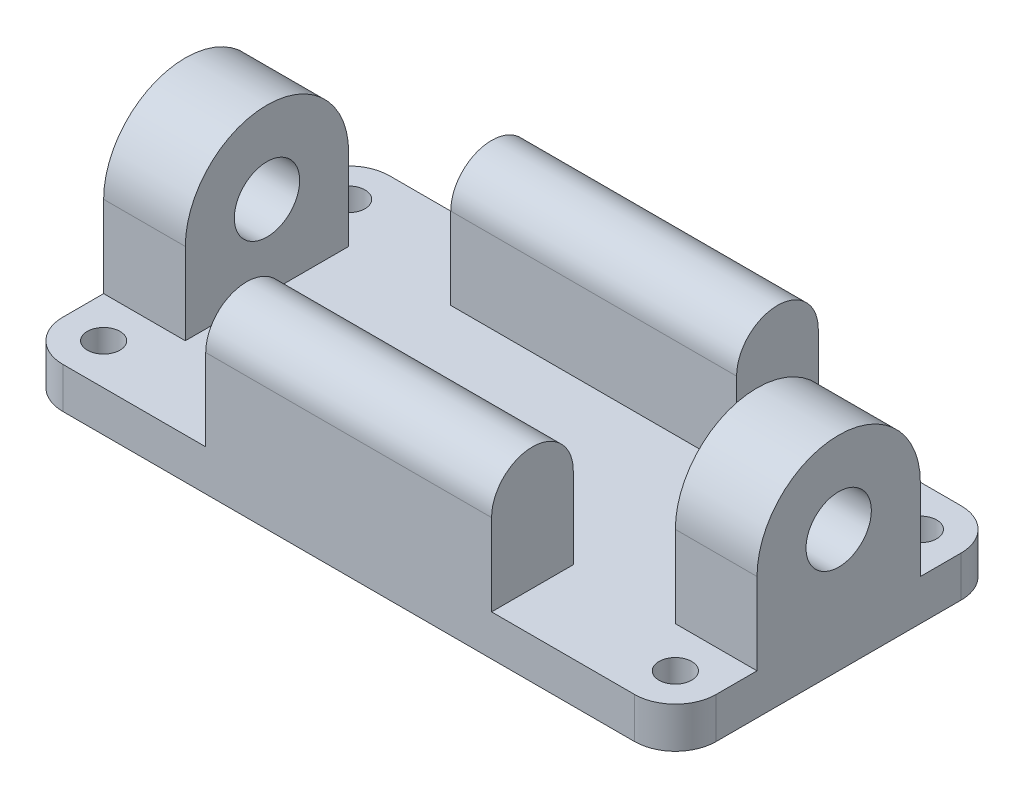
ISO-10303-21;
HEADER;
FILE_DESCRIPTION(('STEP AP214'),'2;1');
FILE_NAME('part.step','',(''),(''),'','','');
FILE_SCHEMA(('AUTOMOTIVE_DESIGN { 1 0 10303 214 1 1 1 1 }'));
ENDSEC;
DATA;
#1=APPLICATION_CONTEXT('core data for automotive mechanical design processes');
#2=APPLICATION_PROTOCOL_DEFINITION('international standard','automotive_design',2000,#1);
#3=PRODUCT_CONTEXT('',#1,'mechanical');
#4=PRODUCT('Part','Part','',(#3));
#5=PRODUCT_RELATED_PRODUCT_CATEGORY('part','',(#4));
#6=PRODUCT_DEFINITION_FORMATION('','',#4);
#7=PRODUCT_DEFINITION_CONTEXT('part definition',#1,'design');
#8=PRODUCT_DEFINITION('design','',#6,#7);
#9=PRODUCT_DEFINITION_SHAPE('','',#8);
#10=(LENGTH_UNIT() NAMED_UNIT(*) SI_UNIT(.MILLI.,.METRE.));
#11=(NAMED_UNIT(*) PLANE_ANGLE_UNIT() SI_UNIT($,.RADIAN.));
#12=(NAMED_UNIT(*) SI_UNIT($,.STERADIAN.) SOLID_ANGLE_UNIT());
#13=UNCERTAINTY_MEASURE_WITH_UNIT(LENGTH_MEASURE(1.E-05),#10,'distance_accuracy_value','');
#14=(GEOMETRIC_REPRESENTATION_CONTEXT(3) GLOBAL_UNCERTAINTY_ASSIGNED_CONTEXT((#13)) GLOBAL_UNIT_ASSIGNED_CONTEXT((#10,
#11,#12)) REPRESENTATION_CONTEXT('',''));
#15=CARTESIAN_POINT('',(0.,0.,0.));
#16=DIRECTION('',(0.,0.,1.));
#17=DIRECTION('',(1.,0.,0.));
#18=AXIS2_PLACEMENT_3D('',#15,#16,#17);
#19=CARTESIAN_POINT('',(35.,5.,-15.));
#20=DIRECTION('',(0.,-1.,0.));
#21=DIRECTION('',(0.,0.,-1.));
#22=AXIS2_PLACEMENT_3D('',#19,#20,#21);
#23=PLANE('',#22);
#24=CARTESIAN_POINT('',(-35.,5.,-15.));
#25=DIRECTION('',(0.,1.,0.));
#26=DIRECTION('',(0.,0.,1.));
#27=AXIS2_PLACEMENT_3D('',#24,#25,#26);
#28=CIRCLE('',#27,1.99999999999999);
#29=CARTESIAN_POINT('',(-35.,5.,-13.));
#30=VERTEX_POINT('',#29);
#31=EDGE_CURVE('E328',#30,#30,#28,.T.);
#32=ORIENTED_EDGE('',*,*,#31,.F.);
#33=EDGE_LOOP('',(#32));
#34=FACE_BOUND('',#33,.T.);
#35=CARTESIAN_POINT('',(35.,5.,-15.));
#36=DIRECTION('',(0.,1.,0.));
#37=DIRECTION('',(0.,0.,1.));
#38=AXIS2_PLACEMENT_3D('',#35,#36,#37);
#39=CIRCLE('',#38,1.99999999999999);
#40=CARTESIAN_POINT('',(35.,5.,-13.));
#41=VERTEX_POINT('',#40);
#42=EDGE_CURVE('E341',#41,#41,#39,.T.);
#43=ORIENTED_EDGE('',*,*,#42,.F.);
#44=EDGE_LOOP('',(#43));
#45=FACE_BOUND('',#44,.T.);
#46=CARTESIAN_POINT('',(35.,5.,15.));
#47=DIRECTION('',(0.,1.,0.));
#48=DIRECTION('',(0.,0.,1.));
#49=AXIS2_PLACEMENT_3D('',#46,#47,#48);
#50=CIRCLE('',#49,1.99999999999999);
#51=CARTESIAN_POINT('',(35.,5.,17.));
#52=VERTEX_POINT('',#51);
#53=EDGE_CURVE('E350',#52,#52,#50,.T.);
#54=ORIENTED_EDGE('',*,*,#53,.F.);
#55=EDGE_LOOP('',(#54));
#56=FACE_BOUND('',#55,.T.);
#57=CARTESIAN_POINT('',(-35.,5.,15.));
#58=DIRECTION('',(0.,1.,0.));
#59=DIRECTION('',(0.,0.,1.));
#60=AXIS2_PLACEMENT_3D('',#57,#58,#59);
#61=CIRCLE('',#60,1.99999999999999);
#62=CARTESIAN_POINT('',(-35.,5.,17.));
#63=VERTEX_POINT('',#62);
#64=EDGE_CURVE('E353',#63,#63,#61,.T.);
#65=ORIENTED_EDGE('',*,*,#64,.F.);
#66=EDGE_LOOP('',(#65));
#67=FACE_BOUND('',#66,.T.);
#68=DIRECTION('',(-1.,0.,0.));
#69=VECTOR('',#68,1.);
#70=CARTESIAN_POINT('',(-35.,5.,-20.));
#71=LINE('',#70,#69);
#72=CARTESIAN_POINT('',(35.,5.,-20.));
#73=VERTEX_POINT('',#72);
#74=CARTESIAN_POINT('',(17.5,5.,-20.));
#75=VERTEX_POINT('',#74);
#76=EDGE_CURVE('E364',#73,#75,#71,.T.);
#77=ORIENTED_EDGE('',*,*,#76,.T.);
#78=DIRECTION('',(0.,0.,1.));
#79=VECTOR('',#78,1.);
#80=CARTESIAN_POINT('',(17.5,5.,-9.99999999999999));
#81=LINE('',#80,#79);
#82=CARTESIAN_POINT('',(17.5,5.,-9.99999999999999));
#83=VERTEX_POINT('',#82);
#84=EDGE_CURVE('E53',#75,#83,#81,.T.);
#85=ORIENTED_EDGE('',*,*,#84,.T.);
#86=DIRECTION('',(-1.,0.,0.));
#87=VECTOR('',#86,1.);
#88=CARTESIAN_POINT('',(17.5,5.,-9.99999999999999));
#89=LINE('',#88,#87);
#90=CARTESIAN_POINT('',(-17.5,5.,-9.99999999999999));
#91=VERTEX_POINT('',#90);
#92=EDGE_CURVE('E59',#83,#91,#89,.T.);
#93=ORIENTED_EDGE('',*,*,#92,.T.);
#94=DIRECTION('',(0.,0.,1.));
#95=VECTOR('',#94,1.);
#96=CARTESIAN_POINT('',(-17.5,5.,-9.99999999999999));
#97=LINE('',#96,#95);
#98=CARTESIAN_POINT('',(-17.5,5.,-20.));
#99=VERTEX_POINT('',#98);
#100=EDGE_CURVE('E223',#99,#91,#97,.T.);
#101=ORIENTED_EDGE('',*,*,#100,.F.);
#102=CARTESIAN_POINT('',(-35.,5.,-20.));
#103=VERTEX_POINT('',#102);
#104=EDGE_CURVE('E361',#99,#103,#71,.T.);
#105=ORIENTED_EDGE('',*,*,#104,.T.);
#106=CARTESIAN_POINT('',(-35.,5.,-15.));
#107=DIRECTION('',(0.,1.,0.));
#108=DIRECTION('',(0.,0.,-1.));
#109=AXIS2_PLACEMENT_3D('',#106,#107,#108);
#110=CIRCLE('',#109,5.);
#111=CARTESIAN_POINT('',(-40.,5.,-15.));
#112=VERTEX_POINT('',#111);
#113=EDGE_CURVE('E370',#103,#112,#110,.T.);
#114=ORIENTED_EDGE('',*,*,#113,.T.);
#115=DIRECTION('',(0.,0.,1.));
#116=VECTOR('',#115,1.);
#117=CARTESIAN_POINT('',(-40.,5.,15.));
#118=LINE('',#117,#116);
#119=CARTESIAN_POINT('',(-40.,5.,-10.));
#120=VERTEX_POINT('',#119);
#121=EDGE_CURVE('E367',#112,#120,#118,.T.);
#122=ORIENTED_EDGE('',*,*,#121,.T.);
#123=DIRECTION('',(-1.,0.,0.));
#124=VECTOR('',#123,1.);
#125=CARTESIAN_POINT('',(-30.,5.,-10.));
#126=LINE('',#125,#124);
#127=CARTESIAN_POINT('',(-30.,5.,-10.));
#128=VERTEX_POINT('',#127);
#129=EDGE_CURVE('E293',#128,#120,#126,.T.);
#130=ORIENTED_EDGE('',*,*,#129,.F.);
#131=DIRECTION('',(0.,0.,-1.));
#132=VECTOR('',#131,1.);
#133=CARTESIAN_POINT('',(-30.,5.,9.99999999999999));
#134=LINE('',#133,#132);
#135=CARTESIAN_POINT('',(-30.,5.,10.));
#136=VERTEX_POINT('',#135);
#137=EDGE_CURVE('E274',#136,#128,#134,.T.);
#138=ORIENTED_EDGE('',*,*,#137,.F.);
#139=DIRECTION('',(-1.,0.,0.));
#140=VECTOR('',#139,1.);
#141=CARTESIAN_POINT('',(-30.,5.,9.99999999999999));
#142=LINE('',#141,#140);
#143=CARTESIAN_POINT('',(-40.,5.,9.99999999999999));
#144=VERTEX_POINT('',#143);
#145=EDGE_CURVE('E295',#136,#144,#142,.T.);
#146=ORIENTED_EDGE('',*,*,#145,.T.);
#147=CARTESIAN_POINT('',(-40.,5.,15.));
#148=VERTEX_POINT('',#147);
#149=EDGE_CURVE('E369',#144,#148,#118,.T.);
#150=ORIENTED_EDGE('',*,*,#149,.T.);
#151=CARTESIAN_POINT('',(-35.,5.,15.));
#152=DIRECTION('',(0.,1.,0.));
#153=DIRECTION('',(0.,0.,-1.));
#154=AXIS2_PLACEMENT_3D('',#151,#152,#153);
#155=CIRCLE('',#154,5.);
#156=CARTESIAN_POINT('',(-35.,5.,20.));
#157=VERTEX_POINT('',#156);
#158=EDGE_CURVE('E375',#148,#157,#155,.T.);
#159=ORIENTED_EDGE('',*,*,#158,.T.);
#160=DIRECTION('',(1.,0.,0.));
#161=VECTOR('',#160,1.);
#162=CARTESIAN_POINT('',(-35.,5.,20.));
#163=LINE('',#162,#161);
#164=CARTESIAN_POINT('',(-17.5,5.,20.));
#165=VERTEX_POINT('',#164);
#166=EDGE_CURVE('E374',#157,#165,#163,.T.);
#167=ORIENTED_EDGE('',*,*,#166,.T.);
#168=DIRECTION('',(0.,0.,-1.));
#169=VECTOR('',#168,1.);
#170=CARTESIAN_POINT('',(-17.5,5.,9.99999999999999));
#171=LINE('',#170,#169);
#172=CARTESIAN_POINT('',(-17.5,5.,10.));
#173=VERTEX_POINT('',#172);
#174=EDGE_CURVE('E207',#165,#173,#171,.T.);
#175=ORIENTED_EDGE('',*,*,#174,.T.);
#176=DIRECTION('',(-1.,0.,0.));
#177=VECTOR('',#176,1.);
#178=CARTESIAN_POINT('',(17.5,5.,9.99999999999999));
#179=LINE('',#178,#177);
#180=CARTESIAN_POINT('',(17.5,5.,10.));
#181=VERTEX_POINT('',#180);
#182=EDGE_CURVE('E259',#181,#173,#179,.T.);
#183=ORIENTED_EDGE('',*,*,#182,.F.);
#184=DIRECTION('',(0.,0.,-1.));
#185=VECTOR('',#184,1.);
#186=CARTESIAN_POINT('',(17.5,5.,9.99999999999999));
#187=LINE('',#186,#185);
#188=CARTESIAN_POINT('',(17.5,5.,20.));
#189=VERTEX_POINT('',#188);
#190=EDGE_CURVE('E234',#189,#181,#187,.T.);
#191=ORIENTED_EDGE('',*,*,#190,.F.);
#192=CARTESIAN_POINT('',(35.,5.,20.));
#193=VERTEX_POINT('',#192);
#194=EDGE_CURVE('E372',#189,#193,#163,.T.);
#195=ORIENTED_EDGE('',*,*,#194,.T.);
#196=CARTESIAN_POINT('',(35.,5.,15.));
#197=DIRECTION('',(0.,1.,0.));
#198=DIRECTION('',(0.,0.,1.));
#199=AXIS2_PLACEMENT_3D('',#196,#197,#198);
#200=CIRCLE('',#199,5.);
#201=CARTESIAN_POINT('',(40.,5.,15.));
#202=VERTEX_POINT('',#201);
#203=EDGE_CURVE('E380',#193,#202,#200,.T.);
#204=ORIENTED_EDGE('',*,*,#203,.T.);
#205=DIRECTION('',(0.,0.,-1.));
#206=VECTOR('',#205,1.);
#207=CARTESIAN_POINT('',(40.,5.,15.));
#208=LINE('',#207,#206);
#209=CARTESIAN_POINT('',(40.,5.,9.99999999999999));
#210=VERTEX_POINT('',#209);
#211=EDGE_CURVE('E379',#202,#210,#208,.T.);
#212=ORIENTED_EDGE('',*,*,#211,.T.);
#213=DIRECTION('',(1.,0.,0.));
#214=VECTOR('',#213,1.);
#215=CARTESIAN_POINT('',(30.,5.,9.99999999999999));
#216=LINE('',#215,#214);
#217=CARTESIAN_POINT('',(30.,5.,9.99999999999999));
#218=VERTEX_POINT('',#217);
#219=EDGE_CURVE('E334',#218,#210,#216,.T.);
#220=ORIENTED_EDGE('',*,*,#219,.F.);
#221=DIRECTION('',(0.,0.,-1.));
#222=VECTOR('',#221,1.);
#223=CARTESIAN_POINT('',(30.,5.,9.99999999999999));
#224=LINE('',#223,#222);
#225=CARTESIAN_POINT('',(30.,5.,-10.));
#226=VERTEX_POINT('',#225);
#227=EDGE_CURVE('E311',#218,#226,#224,.T.);
#228=ORIENTED_EDGE('',*,*,#227,.T.);
#229=DIRECTION('',(1.,0.,0.));
#230=VECTOR('',#229,1.);
#231=CARTESIAN_POINT('',(30.,5.,-10.));
#232=LINE('',#231,#230);
#233=CARTESIAN_POINT('',(40.,5.,-10.));
#234=VERTEX_POINT('',#233);
#235=EDGE_CURVE('E329',#226,#234,#232,.T.);
#236=ORIENTED_EDGE('',*,*,#235,.T.);
#237=CARTESIAN_POINT('',(40.,5.,-15.));
#238=VERTEX_POINT('',#237);
#239=EDGE_CURVE('E377',#234,#238,#208,.T.);
#240=ORIENTED_EDGE('',*,*,#239,.T.);
#241=CARTESIAN_POINT('',(35.,5.,-15.));
#242=DIRECTION('',(0.,1.,0.));
#243=DIRECTION('',(0.,0.,-1.));
#244=AXIS2_PLACEMENT_3D('',#241,#242,#243);
#245=CIRCLE('',#244,5.);
#246=EDGE_CURVE('E359',#238,#73,#245,.T.);
#247=ORIENTED_EDGE('',*,*,#246,.T.);
#248=EDGE_LOOP('',(#77,#85,#93,#101,#105,#114,#122,#130,#138,#146,#150,#159,#167,#175,#183,#191,
#195,#204,#212,#220,#228,#236,#240,#247));
#249=FACE_BOUND('',#248,.T.);
#250=ADVANCED_FACE('F39',(#34,#45,#56,#67,#249),#23,.F.);
#251=CARTESIAN_POINT('',(35.,5.,-15.));
#252=DIRECTION('',(0.,-1.,0.));
#253=DIRECTION('',(0.,0.,-1.));
#254=AXIS2_PLACEMENT_3D('',#251,#252,#253);
#255=CYLINDRICAL_SURFACE('',#254,5.);
#256=CARTESIAN_POINT('',(35.,0.,-15.));
#257=DIRECTION('',(0.,1.,0.));
#258=DIRECTION('',(0.,0.,-1.));
#259=AXIS2_PLACEMENT_3D('',#256,#257,#258);
#260=CIRCLE('',#259,5.);
#261=CARTESIAN_POINT('',(40.,0.,-15.));
#262=VERTEX_POINT('',#261);
#263=CARTESIAN_POINT('',(35.,0.,-20.));
#264=VERTEX_POINT('',#263);
#265=EDGE_CURVE('E358',#262,#264,#260,.T.);
#266=ORIENTED_EDGE('',*,*,#265,.T.);
#267=DIRECTION('',(0.,-1.,0.));
#268=VECTOR('',#267,1.);
#269=CARTESIAN_POINT('',(35.,5.,-20.));
#270=LINE('',#269,#268);
#271=EDGE_CURVE('E11',#73,#264,#270,.T.);
#272=ORIENTED_EDGE('',*,*,#271,.F.);
#273=ORIENTED_EDGE('',*,*,#246,.F.);
#274=DIRECTION('',(0.,-1.,0.));
#275=VECTOR('',#274,1.);
#276=CARTESIAN_POINT('',(40.,5.,-15.));
#277=LINE('',#276,#275);
#278=EDGE_CURVE('E382',#238,#262,#277,.T.);
#279=ORIENTED_EDGE('',*,*,#278,.T.);
#280=EDGE_LOOP('',(#266,#272,#273,#279));
#281=FACE_BOUND('',#280,.T.);
#282=ADVANCED_FACE('F41',(#281),#255,.T.);
#283=CARTESIAN_POINT('',(-35.,5.,-20.));
#284=DIRECTION('',(0.,0.,1.));
#285=DIRECTION('',(1.,0.,0.));
#286=AXIS2_PLACEMENT_3D('',#283,#284,#285);
#287=PLANE('',#286);
#288=DIRECTION('',(-1.,0.,0.));
#289=VECTOR('',#288,1.);
#290=CARTESIAN_POINT('',(-35.,0.,-20.));
#291=LINE('',#290,#289);
#292=CARTESIAN_POINT('',(-35.,0.,-20.));
#293=VERTEX_POINT('',#292);
#294=EDGE_CURVE('E387',#264,#293,#291,.T.);
#295=ORIENTED_EDGE('',*,*,#294,.T.);
#296=DIRECTION('',(0.,-1.,0.));
#297=VECTOR('',#296,1.);
#298=CARTESIAN_POINT('',(-35.,5.,-20.));
#299=LINE('',#298,#297);
#300=EDGE_CURVE('E50',#103,#293,#299,.T.);
#301=ORIENTED_EDGE('',*,*,#300,.F.);
#302=ORIENTED_EDGE('',*,*,#104,.F.);
#303=DIRECTION('',(0.,-1.,0.));
#304=VECTOR('',#303,1.);
#305=CARTESIAN_POINT('',(-17.5,5.,-20.));
#306=LINE('',#305,#304);
#307=CARTESIAN_POINT('',(-17.5,15.,-20.));
#308=VERTEX_POINT('',#307);
#309=EDGE_CURVE('E204',#308,#99,#306,.T.);
#310=ORIENTED_EDGE('',*,*,#309,.F.);
#311=DIRECTION('',(-1.,0.,0.));
#312=VECTOR('',#311,1.);
#313=CARTESIAN_POINT('',(17.5,15.,-20.));
#314=LINE('',#313,#312);
#315=CARTESIAN_POINT('',(17.5,15.,-20.));
#316=VERTEX_POINT('',#315);
#317=EDGE_CURVE('E200',#316,#308,#314,.T.);
#318=ORIENTED_EDGE('',*,*,#317,.F.);
#319=DIRECTION('',(0.,-1.,0.));
#320=VECTOR('',#319,1.);
#321=CARTESIAN_POINT('',(17.5,5.,-20.));
#322=LINE('',#321,#320);
#323=EDGE_CURVE('E205',#316,#75,#322,.T.);
#324=ORIENTED_EDGE('',*,*,#323,.T.);
#325=ORIENTED_EDGE('',*,*,#76,.F.);
#326=ORIENTED_EDGE('',*,*,#271,.T.);
#327=EDGE_LOOP('',(#295,#301,#302,#310,#318,#324,#325,#326));
#328=FACE_BOUND('',#327,.T.);
#329=ADVANCED_FACE('F203',(#328),#287,.F.);
#330=CARTESIAN_POINT('',(-35.,5.,-15.));
#331=DIRECTION('',(0.,-1.,0.));
#332=DIRECTION('',(0.,0.,-1.));
#333=AXIS2_PLACEMENT_3D('',#330,#331,#332);
#334=CYLINDRICAL_SURFACE('',#333,5.);
#335=CARTESIAN_POINT('',(-35.,0.,-15.));
#336=DIRECTION('',(0.,1.,0.));
#337=DIRECTION('',(0.,0.,-1.));
#338=AXIS2_PLACEMENT_3D('',#335,#336,#337);
#339=CIRCLE('',#338,5.);
#340=CARTESIAN_POINT('',(-40.,0.,-15.));
#341=VERTEX_POINT('',#340);
#342=EDGE_CURVE('E389',#293,#341,#339,.T.);
#343=ORIENTED_EDGE('',*,*,#342,.T.);
#344=DIRECTION('',(0.,-1.,0.));
#345=VECTOR('',#344,1.);
#346=CARTESIAN_POINT('',(-40.,5.,-15.));
#347=LINE('',#346,#345);
#348=EDGE_CURVE('E412',#112,#341,#347,.T.);
#349=ORIENTED_EDGE('',*,*,#348,.F.);
#350=ORIENTED_EDGE('',*,*,#113,.F.);
#351=ORIENTED_EDGE('',*,*,#300,.T.);
#352=EDGE_LOOP('',(#343,#349,#350,#351));
#353=FACE_BOUND('',#352,.T.);
#354=ADVANCED_FACE('F419',(#353),#334,.T.);
#355=CARTESIAN_POINT('',(-40.,5.,15.));
#356=DIRECTION('',(1.,0.,0.));
#357=DIRECTION('',(0.,0.,-1.));
#358=AXIS2_PLACEMENT_3D('',#355,#356,#357);
#359=PLANE('',#358);
#360=DIRECTION('',(0.,0.,1.));
#361=VECTOR('',#360,1.);
#362=CARTESIAN_POINT('',(-40.,0.,15.));
#363=LINE('',#362,#361);
#364=CARTESIAN_POINT('',(-40.,0.,15.));
#365=VERTEX_POINT('',#364);
#366=EDGE_CURVE('E388',#341,#365,#363,.T.);
#367=ORIENTED_EDGE('',*,*,#366,.T.);
#368=DIRECTION('',(0.,-1.,0.));
#369=VECTOR('',#368,1.);
#370=CARTESIAN_POINT('',(-40.,5.,15.));
#371=LINE('',#370,#369);
#372=EDGE_CURVE('E406',#148,#365,#371,.T.);
#373=ORIENTED_EDGE('',*,*,#372,.F.);
#374=ORIENTED_EDGE('',*,*,#149,.F.);
#375=DIRECTION('',(0.,-1.,0.));
#376=VECTOR('',#375,1.);
#377=CARTESIAN_POINT('',(-40.,15.,10.));
#378=LINE('',#377,#376);
#379=CARTESIAN_POINT('',(-40.,15.,10.));
#380=VERTEX_POINT('',#379);
#381=EDGE_CURVE('E272',#380,#144,#378,.T.);
#382=ORIENTED_EDGE('',*,*,#381,.F.);
#383=CARTESIAN_POINT('',(-40.,15.,0.));
#384=DIRECTION('',(1.,0.,0.));
#385=DIRECTION('',(0.,0.,-1.));
#386=AXIS2_PLACEMENT_3D('',#383,#384,#385);
#387=CIRCLE('',#386,10.);
#388=CARTESIAN_POINT('',(-40.,15.,-10.));
#389=VERTEX_POINT('',#388);
#390=EDGE_CURVE('E266',#389,#380,#387,.T.);
#391=ORIENTED_EDGE('',*,*,#390,.F.);
#392=DIRECTION('',(0.,1.,0.));
#393=VECTOR('',#392,1.);
#394=CARTESIAN_POINT('',(-40.,5.,-10.));
#395=LINE('',#394,#393);
#396=EDGE_CURVE('E284',#120,#389,#395,.T.);
#397=ORIENTED_EDGE('',*,*,#396,.F.);
#398=ORIENTED_EDGE('',*,*,#121,.F.);
#399=ORIENTED_EDGE('',*,*,#348,.T.);
#400=EDGE_LOOP('',(#367,#373,#374,#382,#391,#397,#398,#399));
#401=FACE_BOUND('',#400,.T.);
#402=CARTESIAN_POINT('',(-40.,15.,0.));
#403=DIRECTION('',(1.,0.,0.));
#404=DIRECTION('',(0.,0.,-1.));
#405=AXIS2_PLACEMENT_3D('',#402,#403,#404);
#406=CIRCLE('',#405,4.);
#407=CARTESIAN_POINT('',(-40.,15.,-4.00000000000001));
#408=VERTEX_POINT('',#407);
#409=EDGE_CURVE('E265',#408,#408,#406,.T.);
#410=ORIENTED_EDGE('',*,*,#409,.T.);
#411=EDGE_LOOP('',(#410));
#412=FACE_BOUND('',#411,.T.);
#413=ADVANCED_FACE('F429',(#401,#412),#359,.F.);
#414=CARTESIAN_POINT('',(-35.,5.,15.));
#415=DIRECTION('',(0.,-1.,0.));
#416=DIRECTION('',(0.,0.,-1.));
#417=AXIS2_PLACEMENT_3D('',#414,#415,#416);
#418=CYLINDRICAL_SURFACE('',#417,5.);
#419=CARTESIAN_POINT('',(-35.,0.,15.));
#420=DIRECTION('',(0.,1.,0.));
#421=DIRECTION('',(0.,0.,-1.));
#422=AXIS2_PLACEMENT_3D('',#419,#420,#421);
#423=CIRCLE('',#422,5.);
#424=CARTESIAN_POINT('',(-35.,0.,20.));
#425=VERTEX_POINT('',#424);
#426=EDGE_CURVE('E395',#365,#425,#423,.T.);
#427=ORIENTED_EDGE('',*,*,#426,.T.);
#428=DIRECTION('',(0.,-1.,0.));
#429=VECTOR('',#428,1.);
#430=CARTESIAN_POINT('',(-35.,5.,20.));
#431=LINE('',#430,#429);
#432=EDGE_CURVE('E410',#157,#425,#431,.T.);
#433=ORIENTED_EDGE('',*,*,#432,.F.);
#434=ORIENTED_EDGE('',*,*,#158,.F.);
#435=ORIENTED_EDGE('',*,*,#372,.T.);
#436=EDGE_LOOP('',(#427,#433,#434,#435));
#437=FACE_BOUND('',#436,.T.);
#438=ADVANCED_FACE('F434',(#437),#418,.T.);
#439=CARTESIAN_POINT('',(-35.,5.,20.));
#440=DIRECTION('',(0.,0.,-1.));
#441=DIRECTION('',(-1.,0.,0.));
#442=AXIS2_PLACEMENT_3D('',#439,#440,#441);
#443=PLANE('',#442);
#444=DIRECTION('',(1.,0.,0.));
#445=VECTOR('',#444,1.);
#446=CARTESIAN_POINT('',(-35.,0.,20.));
#447=LINE('',#446,#445);
#448=CARTESIAN_POINT('',(35.,0.,20.));
#449=VERTEX_POINT('',#448);
#450=EDGE_CURVE('E394',#425,#449,#447,.T.);
#451=ORIENTED_EDGE('',*,*,#450,.T.);
#452=DIRECTION('',(0.,-1.,0.));
#453=VECTOR('',#452,1.);
#454=CARTESIAN_POINT('',(35.,5.,20.));
#455=LINE('',#454,#453);
#456=EDGE_CURVE('E404',#193,#449,#455,.T.);
#457=ORIENTED_EDGE('',*,*,#456,.F.);
#458=ORIENTED_EDGE('',*,*,#194,.F.);
#459=DIRECTION('',(0.,-1.,0.));
#460=VECTOR('',#459,1.);
#461=CARTESIAN_POINT('',(17.5,5.,20.));
#462=LINE('',#461,#460);
#463=CARTESIAN_POINT('',(17.5,15.,20.));
#464=VERTEX_POINT('',#463);
#465=EDGE_CURVE('E243',#464,#189,#462,.T.);
#466=ORIENTED_EDGE('',*,*,#465,.F.);
#467=DIRECTION('',(-1.,0.,0.));
#468=VECTOR('',#467,1.);
#469=CARTESIAN_POINT('',(17.5,15.,20.));
#470=LINE('',#469,#468);
#471=CARTESIAN_POINT('',(-17.5,15.,20.));
#472=VERTEX_POINT('',#471);
#473=EDGE_CURVE('E246',#464,#472,#470,.T.);
#474=ORIENTED_EDGE('',*,*,#473,.T.);
#475=DIRECTION('',(0.,-1.,0.));
#476=VECTOR('',#475,1.);
#477=CARTESIAN_POINT('',(-17.5,5.,20.));
#478=LINE('',#477,#476);
#479=EDGE_CURVE('E239',#472,#165,#478,.T.);
#480=ORIENTED_EDGE('',*,*,#479,.T.);
#481=ORIENTED_EDGE('',*,*,#166,.F.);
#482=ORIENTED_EDGE('',*,*,#432,.T.);
#483=EDGE_LOOP('',(#451,#457,#458,#466,#474,#480,#481,#482));
#484=FACE_BOUND('',#483,.T.);
#485=ADVANCED_FACE('F491',(#484),#443,.F.);
#486=CARTESIAN_POINT('',(35.,5.,15.));
#487=DIRECTION('',(0.,-1.,0.));
#488=DIRECTION('',(0.,0.,-1.));
#489=AXIS2_PLACEMENT_3D('',#486,#487,#488);
#490=CYLINDRICAL_SURFACE('',#489,5.);
#491=CARTESIAN_POINT('',(35.,0.,15.));
#492=DIRECTION('',(0.,1.,0.));
#493=DIRECTION('',(0.,0.,1.));
#494=AXIS2_PLACEMENT_3D('',#491,#492,#493);
#495=CIRCLE('',#494,5.);
#496=CARTESIAN_POINT('',(40.,0.,15.));
#497=VERTEX_POINT('',#496);
#498=EDGE_CURVE('E396',#449,#497,#495,.T.);
#499=ORIENTED_EDGE('',*,*,#498,.T.);
#500=DIRECTION('',(0.,-1.,0.));
#501=VECTOR('',#500,1.);
#502=CARTESIAN_POINT('',(40.,5.,15.));
#503=LINE('',#502,#501);
#504=EDGE_CURVE('E402',#202,#497,#503,.T.);
#505=ORIENTED_EDGE('',*,*,#504,.F.);
#506=ORIENTED_EDGE('',*,*,#203,.F.);
#507=ORIENTED_EDGE('',*,*,#456,.T.);
#508=EDGE_LOOP('',(#499,#505,#506,#507));
#509=FACE_BOUND('',#508,.T.);
#510=ADVANCED_FACE('F490',(#509),#490,.T.);
#511=CARTESIAN_POINT('',(40.,5.,15.));
#512=DIRECTION('',(-1.,0.,0.));
#513=DIRECTION('',(0.,0.,1.));
#514=AXIS2_PLACEMENT_3D('',#511,#512,#513);
#515=PLANE('',#514);
#516=DIRECTION('',(0.,0.,-1.));
#517=VECTOR('',#516,1.);
#518=CARTESIAN_POINT('',(40.,0.,15.));
#519=LINE('',#518,#517);
#520=EDGE_CURVE('E365',#497,#262,#519,.T.);
#521=ORIENTED_EDGE('',*,*,#520,.T.);
#522=ORIENTED_EDGE('',*,*,#278,.F.);
#523=ORIENTED_EDGE('',*,*,#239,.F.);
#524=DIRECTION('',(0.,1.,0.));
#525=VECTOR('',#524,1.);
#526=CARTESIAN_POINT('',(40.,5.,-10.));
#527=LINE('',#526,#525);
#528=CARTESIAN_POINT('',(40.,15.,-10.));
#529=VERTEX_POINT('',#528);
#530=EDGE_CURVE('E309',#234,#529,#527,.T.);
#531=ORIENTED_EDGE('',*,*,#530,.T.);
#532=CARTESIAN_POINT('',(40.,15.,0.));
#533=DIRECTION('',(1.,0.,0.));
#534=DIRECTION('',(0.,0.,-1.));
#535=AXIS2_PLACEMENT_3D('',#532,#533,#534);
#536=CIRCLE('',#535,10.);
#537=CARTESIAN_POINT('',(40.,15.,10.));
#538=VERTEX_POINT('',#537);
#539=EDGE_CURVE('E302',#529,#538,#536,.T.);
#540=ORIENTED_EDGE('',*,*,#539,.T.);
#541=DIRECTION('',(0.,-1.,0.));
#542=VECTOR('',#541,1.);
#543=CARTESIAN_POINT('',(40.,15.,10.));
#544=LINE('',#543,#542);
#545=EDGE_CURVE('E325',#538,#210,#544,.T.);
#546=ORIENTED_EDGE('',*,*,#545,.T.);
#547=ORIENTED_EDGE('',*,*,#211,.F.);
#548=ORIENTED_EDGE('',*,*,#504,.T.);
#549=EDGE_LOOP('',(#521,#522,#523,#531,#540,#546,#547,#548));
#550=FACE_BOUND('',#549,.T.);
#551=CARTESIAN_POINT('',(40.,15.,0.));
#552=DIRECTION('',(1.,0.,0.));
#553=DIRECTION('',(0.,0.,-1.));
#554=AXIS2_PLACEMENT_3D('',#551,#552,#553);
#555=CIRCLE('',#554,4.);
#556=CARTESIAN_POINT('',(40.,15.,-4.00000000000001));
#557=VERTEX_POINT('',#556);
#558=EDGE_CURVE('E292',#557,#557,#555,.T.);
#559=ORIENTED_EDGE('',*,*,#558,.F.);
#560=EDGE_LOOP('',(#559));
#561=FACE_BOUND('',#560,.T.);
#562=ADVANCED_FACE('F483',(#550,#561),#515,.F.);
#563=CARTESIAN_POINT('',(35.,0.,-15.));
#564=DIRECTION('',(0.,-1.,0.));
#565=DIRECTION('',(0.,0.,-1.));
#566=AXIS2_PLACEMENT_3D('',#563,#564,#565);
#567=PLANE('',#566);
#568=CARTESIAN_POINT('',(-35.,0.,-15.));
#569=DIRECTION('',(0.,1.,0.));
#570=DIRECTION('',(0.,0.,1.));
#571=AXIS2_PLACEMENT_3D('',#568,#569,#570);
#572=CIRCLE('',#571,1.99999999999999);
#573=CARTESIAN_POINT('',(-35.,0.,-13.));
#574=VERTEX_POINT('',#573);
#575=EDGE_CURVE('E338',#574,#574,#572,.T.);
#576=ORIENTED_EDGE('',*,*,#575,.T.);
#577=EDGE_LOOP('',(#576));
#578=FACE_BOUND('',#577,.T.);
#579=CARTESIAN_POINT('',(35.,0.,-15.));
#580=DIRECTION('',(0.,1.,0.));
#581=DIRECTION('',(0.,0.,1.));
#582=AXIS2_PLACEMENT_3D('',#579,#580,#581);
#583=CIRCLE('',#582,1.99999999999999);
#584=CARTESIAN_POINT('',(35.,0.,-13.));
#585=VERTEX_POINT('',#584);
#586=EDGE_CURVE('E343',#585,#585,#583,.T.);
#587=ORIENTED_EDGE('',*,*,#586,.T.);
#588=EDGE_LOOP('',(#587));
#589=FACE_BOUND('',#588,.T.);
#590=CARTESIAN_POINT('',(35.,0.,15.));
#591=DIRECTION('',(0.,1.,0.));
#592=DIRECTION('',(0.,0.,1.));
#593=AXIS2_PLACEMENT_3D('',#590,#591,#592);
#594=CIRCLE('',#593,1.99999999999999);
#595=CARTESIAN_POINT('',(35.,0.,17.));
#596=VERTEX_POINT('',#595);
#597=EDGE_CURVE('E348',#596,#596,#594,.T.);
#598=ORIENTED_EDGE('',*,*,#597,.T.);
#599=EDGE_LOOP('',(#598));
#600=FACE_BOUND('',#599,.T.);
#601=CARTESIAN_POINT('',(-35.,0.,15.));
#602=DIRECTION('',(0.,1.,0.));
#603=DIRECTION('',(0.,0.,1.));
#604=AXIS2_PLACEMENT_3D('',#601,#602,#603);
#605=CIRCLE('',#604,1.99999999999999);
#606=CARTESIAN_POINT('',(-35.,0.,17.));
#607=VERTEX_POINT('',#606);
#608=EDGE_CURVE('E356',#607,#607,#605,.T.);
#609=ORIENTED_EDGE('',*,*,#608,.T.);
#610=EDGE_LOOP('',(#609));
#611=FACE_BOUND('',#610,.T.);
#612=ORIENTED_EDGE('',*,*,#265,.F.);
#613=ORIENTED_EDGE('',*,*,#520,.F.);
#614=ORIENTED_EDGE('',*,*,#498,.F.);
#615=ORIENTED_EDGE('',*,*,#450,.F.);
#616=ORIENTED_EDGE('',*,*,#426,.F.);
#617=ORIENTED_EDGE('',*,*,#366,.F.);
#618=ORIENTED_EDGE('',*,*,#342,.F.);
#619=ORIENTED_EDGE('',*,*,#294,.F.);
#620=EDGE_LOOP('',(#612,#613,#614,#615,#616,#617,#618,#619));
#621=FACE_BOUND('',#620,.T.);
#622=ADVANCED_FACE('F422',(#578,#589,#600,#611,#621),#567,.T.);
#623=CARTESIAN_POINT('',(-35.,5.,15.));
#624=DIRECTION('',(0.,1.,0.));
#625=DIRECTION('',(0.,0.,1.));
#626=AXIS2_PLACEMENT_3D('',#623,#624,#625);
#627=CYLINDRICAL_SURFACE('',#626,1.99999999999999);
#628=ORIENTED_EDGE('',*,*,#608,.F.);
#629=EDGE_LOOP('',(#628));
#630=FACE_BOUND('',#629,.T.);
#631=ORIENTED_EDGE('',*,*,#64,.T.);
#632=EDGE_LOOP('',(#631));
#633=FACE_BOUND('',#632,.T.);
#634=ADVANCED_FACE('F479',(#630,#633),#627,.F.);
#635=CARTESIAN_POINT('',(35.,5.,15.));
#636=DIRECTION('',(0.,1.,0.));
#637=DIRECTION('',(0.,0.,1.));
#638=AXIS2_PLACEMENT_3D('',#635,#636,#637);
#639=CYLINDRICAL_SURFACE('',#638,1.99999999999999);
#640=ORIENTED_EDGE('',*,*,#597,.F.);
#641=EDGE_LOOP('',(#640));
#642=FACE_BOUND('',#641,.T.);
#643=ORIENTED_EDGE('',*,*,#53,.T.);
#644=EDGE_LOOP('',(#643));
#645=FACE_BOUND('',#644,.T.);
#646=ADVANCED_FACE('F669',(#642,#645),#639,.F.);
#647=CARTESIAN_POINT('',(35.,5.,-15.));
#648=DIRECTION('',(0.,1.,0.));
#649=DIRECTION('',(0.,0.,1.));
#650=AXIS2_PLACEMENT_3D('',#647,#648,#649);
#651=CYLINDRICAL_SURFACE('',#650,1.99999999999999);
#652=ORIENTED_EDGE('',*,*,#586,.F.);
#653=EDGE_LOOP('',(#652));
#654=FACE_BOUND('',#653,.T.);
#655=ORIENTED_EDGE('',*,*,#42,.T.);
#656=EDGE_LOOP('',(#655));
#657=FACE_BOUND('',#656,.T.);
#658=ADVANCED_FACE('F659',(#654,#657),#651,.F.);
#659=CARTESIAN_POINT('',(-35.,5.,-15.));
#660=DIRECTION('',(0.,1.,0.));
#661=DIRECTION('',(0.,0.,1.));
#662=AXIS2_PLACEMENT_3D('',#659,#660,#661);
#663=CYLINDRICAL_SURFACE('',#662,1.99999999999999);
#664=ORIENTED_EDGE('',*,*,#575,.F.);
#665=EDGE_LOOP('',(#664));
#666=FACE_BOUND('',#665,.T.);
#667=ORIENTED_EDGE('',*,*,#31,.T.);
#668=EDGE_LOOP('',(#667));
#669=FACE_BOUND('',#668,.T.);
#670=ADVANCED_FACE('F649',(#666,#669),#663,.F.);
#671=CARTESIAN_POINT('',(30.,15.,0.));
#672=DIRECTION('',(1.,0.,0.));
#673=DIRECTION('',(0.,0.,-1.));
#674=AXIS2_PLACEMENT_3D('',#671,#672,#673);
#675=CYLINDRICAL_SURFACE('',#674,10.);
#676=ORIENTED_EDGE('',*,*,#539,.F.);
#677=DIRECTION('',(1.,0.,0.));
#678=VECTOR('',#677,1.);
#679=CARTESIAN_POINT('',(30.,15.,-10.));
#680=LINE('',#679,#678);
#681=CARTESIAN_POINT('',(30.,15.,-10.));
#682=VERTEX_POINT('',#681);
#683=EDGE_CURVE('E330',#682,#529,#680,.T.);
#684=ORIENTED_EDGE('',*,*,#683,.F.);
#685=CARTESIAN_POINT('',(30.,15.,0.));
#686=DIRECTION('',(1.,0.,0.));
#687=DIRECTION('',(0.,0.,-1.));
#688=AXIS2_PLACEMENT_3D('',#685,#686,#687);
#689=CIRCLE('',#688,10.);
#690=CARTESIAN_POINT('',(30.,15.,10.));
#691=VERTEX_POINT('',#690);
#692=EDGE_CURVE('E308',#682,#691,#689,.T.);
#693=ORIENTED_EDGE('',*,*,#692,.T.);
#694=DIRECTION('',(1.,0.,0.));
#695=VECTOR('',#694,1.);
#696=CARTESIAN_POINT('',(30.,15.,10.));
#697=LINE('',#696,#695);
#698=EDGE_CURVE('E317',#691,#538,#697,.T.);
#699=ORIENTED_EDGE('',*,*,#698,.T.);
#700=EDGE_LOOP('',(#676,#684,#693,#699));
#701=FACE_BOUND('',#700,.T.);
#702=ADVANCED_FACE('F643',(#701),#675,.T.);
#703=CARTESIAN_POINT('',(30.,5.,-10.));
#704=DIRECTION('',(0.,0.,-1.));
#705=DIRECTION('',(-1.,0.,0.));
#706=AXIS2_PLACEMENT_3D('',#703,#704,#705);
#707=PLANE('',#706);
#708=ORIENTED_EDGE('',*,*,#530,.F.);
#709=ORIENTED_EDGE('',*,*,#235,.F.);
#710=DIRECTION('',(0.,1.,0.));
#711=VECTOR('',#710,1.);
#712=CARTESIAN_POINT('',(30.,5.,-10.));
#713=LINE('',#712,#711);
#714=EDGE_CURVE('E316',#226,#682,#713,.T.);
#715=ORIENTED_EDGE('',*,*,#714,.T.);
#716=ORIENTED_EDGE('',*,*,#683,.T.);
#717=EDGE_LOOP('',(#708,#709,#715,#716));
#718=FACE_BOUND('',#717,.T.);
#719=ADVANCED_FACE('F635',(#718),#707,.T.);
#720=CARTESIAN_POINT('',(30.,15.,10.));
#721=DIRECTION('',(0.,0.,1.));
#722=DIRECTION('',(0.,-1.,0.));
#723=AXIS2_PLACEMENT_3D('',#720,#721,#722);
#724=PLANE('',#723);
#725=ORIENTED_EDGE('',*,*,#545,.F.);
#726=ORIENTED_EDGE('',*,*,#698,.F.);
#727=DIRECTION('',(0.,-1.,0.));
#728=VECTOR('',#727,1.);
#729=CARTESIAN_POINT('',(30.,15.,10.));
#730=LINE('',#729,#728);
#731=EDGE_CURVE('E310',#691,#218,#730,.T.);
#732=ORIENTED_EDGE('',*,*,#731,.T.);
#733=ORIENTED_EDGE('',*,*,#219,.T.);
#734=EDGE_LOOP('',(#725,#726,#732,#733));
#735=FACE_BOUND('',#734,.T.);
#736=ADVANCED_FACE('F621',(#735),#724,.T.);
#737=CARTESIAN_POINT('',(30.,15.,0.));
#738=DIRECTION('',(1.,0.,0.));
#739=DIRECTION('',(0.,0.,-1.));
#740=AXIS2_PLACEMENT_3D('',#737,#738,#739);
#741=PLANE('',#740);
#742=CARTESIAN_POINT('',(30.,15.,0.));
#743=DIRECTION('',(1.,0.,0.));
#744=DIRECTION('',(0.,0.,-1.));
#745=AXIS2_PLACEMENT_3D('',#742,#743,#744);
#746=CIRCLE('',#745,4.);
#747=CARTESIAN_POINT('',(30.,15.,-4.00000000000001));
#748=VERTEX_POINT('',#747);
#749=EDGE_CURVE('E296',#748,#748,#746,.T.);
#750=ORIENTED_EDGE('',*,*,#749,.T.);
#751=EDGE_LOOP('',(#750));
#752=FACE_BOUND('',#751,.T.);
#753=ORIENTED_EDGE('',*,*,#692,.F.);
#754=ORIENTED_EDGE('',*,*,#714,.F.);
#755=ORIENTED_EDGE('',*,*,#227,.F.);
#756=ORIENTED_EDGE('',*,*,#731,.F.);
#757=EDGE_LOOP('',(#753,#754,#755,#756));
#758=FACE_BOUND('',#757,.T.);
#759=ADVANCED_FACE('F614',(#752,#758),#741,.F.);
#760=CARTESIAN_POINT('',(30.,15.,0.));
#761=DIRECTION('',(1.,0.,0.));
#762=DIRECTION('',(0.,0.,-1.));
#763=AXIS2_PLACEMENT_3D('',#760,#761,#762);
#764=CYLINDRICAL_SURFACE('',#763,4.);
#765=ORIENTED_EDGE('',*,*,#749,.F.);
#766=EDGE_LOOP('',(#765));
#767=FACE_BOUND('',#766,.T.);
#768=ORIENTED_EDGE('',*,*,#558,.T.);
#769=EDGE_LOOP('',(#768));
#770=FACE_BOUND('',#769,.T.);
#771=ADVANCED_FACE('F597',(#767,#770),#764,.F.);
#772=CARTESIAN_POINT('',(-30.,15.,0.));
#773=DIRECTION('',(-1.,0.,0.));
#774=DIRECTION('',(0.,0.,-1.));
#775=AXIS2_PLACEMENT_3D('',#772,#773,#774);
#776=PLANE('',#775);
#777=CARTESIAN_POINT('',(-30.,15.,0.));
#778=DIRECTION('',(1.,0.,0.));
#779=DIRECTION('',(0.,0.,-1.));
#780=AXIS2_PLACEMENT_3D('',#777,#778,#779);
#781=CIRCLE('',#780,10.);
#782=CARTESIAN_POINT('',(-30.,15.,-10.));
#783=VERTEX_POINT('',#782);
#784=CARTESIAN_POINT('',(-30.,15.,10.));
#785=VERTEX_POINT('',#784);
#786=EDGE_CURVE('E267',#783,#785,#781,.T.);
#787=ORIENTED_EDGE('',*,*,#786,.T.);
#788=DIRECTION('',(0.,-1.,0.));
#789=VECTOR('',#788,1.);
#790=CARTESIAN_POINT('',(-30.,15.,10.));
#791=LINE('',#790,#789);
#792=EDGE_CURVE('E279',#785,#136,#791,.T.);
#793=ORIENTED_EDGE('',*,*,#792,.T.);
#794=ORIENTED_EDGE('',*,*,#137,.T.);
#795=DIRECTION('',(0.,1.,0.));
#796=VECTOR('',#795,1.);
#797=CARTESIAN_POINT('',(-30.,5.,-10.));
#798=LINE('',#797,#796);
#799=EDGE_CURVE('E275',#128,#783,#798,.T.);
#800=ORIENTED_EDGE('',*,*,#799,.T.);
#801=EDGE_LOOP('',(#787,#793,#794,#800));
#802=FACE_BOUND('',#801,.T.);
#803=CARTESIAN_POINT('',(-30.,15.,0.));
#804=DIRECTION('',(1.,0.,0.));
#805=DIRECTION('',(0.,0.,-1.));
#806=AXIS2_PLACEMENT_3D('',#803,#804,#805);
#807=CIRCLE('',#806,4.);
#808=CARTESIAN_POINT('',(-30.,15.,-4.00000000000001));
#809=VERTEX_POINT('',#808);
#810=EDGE_CURVE('E263',#809,#809,#807,.T.);
#811=ORIENTED_EDGE('',*,*,#810,.F.);
#812=EDGE_LOOP('',(#811));
#813=FACE_BOUND('',#812,.T.);
#814=ADVANCED_FACE('F595',(#802,#813),#776,.F.);
#815=CARTESIAN_POINT('',(-30.,15.,0.));
#816=DIRECTION('',(-1.,0.,0.));
#817=DIRECTION('',(0.,0.,1.));
#818=AXIS2_PLACEMENT_3D('',#815,#816,#817);
#819=CYLINDRICAL_SURFACE('',#818,10.);
#820=ORIENTED_EDGE('',*,*,#390,.T.);
#821=DIRECTION('',(-1.,0.,0.));
#822=VECTOR('',#821,1.);
#823=CARTESIAN_POINT('',(-30.,15.,10.));
#824=LINE('',#823,#822);
#825=EDGE_CURVE('E287',#785,#380,#824,.T.);
#826=ORIENTED_EDGE('',*,*,#825,.F.);
#827=ORIENTED_EDGE('',*,*,#786,.F.);
#828=DIRECTION('',(-1.,0.,0.));
#829=VECTOR('',#828,1.);
#830=CARTESIAN_POINT('',(-30.,15.,-10.));
#831=LINE('',#830,#829);
#832=EDGE_CURVE('E282',#783,#389,#831,.T.);
#833=ORIENTED_EDGE('',*,*,#832,.T.);
#834=EDGE_LOOP('',(#820,#826,#827,#833));
#835=FACE_BOUND('',#834,.T.);
#836=ADVANCED_FACE('F447',(#835),#819,.T.);
#837=CARTESIAN_POINT('',(-30.,15.,10.));
#838=DIRECTION('',(0.,0.,-1.));
#839=DIRECTION('',(0.,1.,0.));
#840=AXIS2_PLACEMENT_3D('',#837,#838,#839);
#841=PLANE('',#840);
#842=ORIENTED_EDGE('',*,*,#381,.T.);
#843=ORIENTED_EDGE('',*,*,#145,.F.);
#844=ORIENTED_EDGE('',*,*,#792,.F.);
#845=ORIENTED_EDGE('',*,*,#825,.T.);
#846=EDGE_LOOP('',(#842,#843,#844,#845));
#847=FACE_BOUND('',#846,.T.);
#848=ADVANCED_FACE('F444',(#847),#841,.F.);
#849=CARTESIAN_POINT('',(-30.,5.,-10.));
#850=DIRECTION('',(0.,0.,1.));
#851=DIRECTION('',(1.,0.,0.));
#852=AXIS2_PLACEMENT_3D('',#849,#850,#851);
#853=PLANE('',#852);
#854=ORIENTED_EDGE('',*,*,#396,.T.);
#855=ORIENTED_EDGE('',*,*,#832,.F.);
#856=ORIENTED_EDGE('',*,*,#799,.F.);
#857=ORIENTED_EDGE('',*,*,#129,.T.);
#858=EDGE_LOOP('',(#854,#855,#856,#857));
#859=FACE_BOUND('',#858,.T.);
#860=ADVANCED_FACE('F446',(#859),#853,.F.);
#861=CARTESIAN_POINT('',(-30.,15.,0.));
#862=DIRECTION('',(-1.,0.,0.));
#863=DIRECTION('',(0.,0.,1.));
#864=AXIS2_PLACEMENT_3D('',#861,#862,#863);
#865=CYLINDRICAL_SURFACE('',#864,4.);
#866=ORIENTED_EDGE('',*,*,#810,.T.);
#867=EDGE_LOOP('',(#866));
#868=FACE_BOUND('',#867,.T.);
#869=ORIENTED_EDGE('',*,*,#409,.F.);
#870=EDGE_LOOP('',(#869));
#871=FACE_BOUND('',#870,.T.);
#872=ADVANCED_FACE('F556',(#868,#871),#865,.F.);
#873=CARTESIAN_POINT('',(17.5,15.,9.99999999999999));
#874=DIRECTION('',(0.,0.,1.));
#875=DIRECTION('',(1.,0.,0.));
#876=AXIS2_PLACEMENT_3D('',#873,#874,#875);
#877=PLANE('',#876);
#878=DIRECTION('',(0.,1.,0.));
#879=VECTOR('',#878,1.);
#880=CARTESIAN_POINT('',(-17.5,15.,9.99999999999999));
#881=LINE('',#880,#879);
#882=CARTESIAN_POINT('',(-17.5,15.,9.99999999999999));
#883=VERTEX_POINT('',#882);
#884=EDGE_CURVE('E247',#173,#883,#881,.T.);
#885=ORIENTED_EDGE('',*,*,#884,.T.);
#886=DIRECTION('',(-1.,0.,0.));
#887=VECTOR('',#886,1.);
#888=CARTESIAN_POINT('',(17.5,15.,9.99999999999999));
#889=LINE('',#888,#887);
#890=CARTESIAN_POINT('',(17.5,15.,9.99999999999999));
#891=VERTEX_POINT('',#890);
#892=EDGE_CURVE('E258',#891,#883,#889,.T.);
#893=ORIENTED_EDGE('',*,*,#892,.F.);
#894=DIRECTION('',(0.,1.,0.));
#895=VECTOR('',#894,1.);
#896=CARTESIAN_POINT('',(17.5,15.,9.99999999999999));
#897=LINE('',#896,#895);
#898=EDGE_CURVE('E236',#181,#891,#897,.T.);
#899=ORIENTED_EDGE('',*,*,#898,.F.);
#900=ORIENTED_EDGE('',*,*,#182,.T.);
#901=EDGE_LOOP('',(#885,#893,#899,#900));
#902=FACE_BOUND('',#901,.T.);
#903=ADVANCED_FACE('F552',(#902),#877,.F.);
#904=CARTESIAN_POINT('',(17.5,15.,15.));
#905=DIRECTION('',(-1.,0.,0.));
#906=DIRECTION('',(0.,0.,1.));
#907=AXIS2_PLACEMENT_3D('',#904,#905,#906);
#908=CYLINDRICAL_SURFACE('',#907,5.);
#909=CARTESIAN_POINT('',(-17.5,15.,15.));
#910=DIRECTION('',(1.,0.,0.));
#911=DIRECTION('',(0.,0.,-1.));
#912=AXIS2_PLACEMENT_3D('',#909,#910,#911);
#913=CIRCLE('',#912,5.);
#914=EDGE_CURVE('E249',#883,#472,#913,.T.);
#915=ORIENTED_EDGE('',*,*,#914,.T.);
#916=ORIENTED_EDGE('',*,*,#473,.F.);
#917=CARTESIAN_POINT('',(17.5,15.,15.));
#918=DIRECTION('',(1.,0.,0.));
#919=DIRECTION('',(0.,0.,-1.));
#920=AXIS2_PLACEMENT_3D('',#917,#918,#919);
#921=CIRCLE('',#920,5.);
#922=EDGE_CURVE('E242',#891,#464,#921,.T.);
#923=ORIENTED_EDGE('',*,*,#922,.F.);
#924=ORIENTED_EDGE('',*,*,#892,.T.);
#925=EDGE_LOOP('',(#915,#916,#923,#924));
#926=FACE_BOUND('',#925,.T.);
#927=ADVANCED_FACE('F545',(#926),#908,.T.);
#928=CARTESIAN_POINT('',(17.5,15.,15.));
#929=DIRECTION('',(1.,0.,0.));
#930=DIRECTION('',(0.,0.,-1.));
#931=AXIS2_PLACEMENT_3D('',#928,#929,#930);
#932=PLANE('',#931);
#933=ORIENTED_EDGE('',*,*,#190,.T.);
#934=ORIENTED_EDGE('',*,*,#898,.T.);
#935=ORIENTED_EDGE('',*,*,#922,.T.);
#936=ORIENTED_EDGE('',*,*,#465,.T.);
#937=EDGE_LOOP('',(#933,#934,#935,#936));
#938=FACE_BOUND('',#937,.T.);
#939=ADVANCED_FACE('F531',(#938),#932,.T.);
#940=CARTESIAN_POINT('',(-17.5,15.,15.));
#941=DIRECTION('',(1.,0.,0.));
#942=DIRECTION('',(0.,0.,-1.));
#943=AXIS2_PLACEMENT_3D('',#940,#941,#942);
#944=PLANE('',#943);
#945=ORIENTED_EDGE('',*,*,#174,.F.);
#946=ORIENTED_EDGE('',*,*,#479,.F.);
#947=ORIENTED_EDGE('',*,*,#914,.F.);
#948=ORIENTED_EDGE('',*,*,#884,.F.);
#949=EDGE_LOOP('',(#945,#946,#947,#948));
#950=FACE_BOUND('',#949,.T.);
#951=ADVANCED_FACE('F463',(#950),#944,.F.);
#952=CARTESIAN_POINT('',(17.5,15.,-15.));
#953=DIRECTION('',(-1.,0.,0.));
#954=DIRECTION('',(0.,0.,1.));
#955=AXIS2_PLACEMENT_3D('',#952,#953,#954);
#956=CYLINDRICAL_SURFACE('',#955,5.);
#957=CARTESIAN_POINT('',(-17.5,15.,-15.));
#958=DIRECTION('',(-1.,0.,0.));
#959=DIRECTION('',(0.,0.,1.));
#960=AXIS2_PLACEMENT_3D('',#957,#958,#959);
#961=CIRCLE('',#960,5.);
#962=CARTESIAN_POINT('',(-17.5,15.,-9.99999999999999));
#963=VERTEX_POINT('',#962);
#964=EDGE_CURVE('E228',#963,#308,#961,.T.);
#965=ORIENTED_EDGE('',*,*,#964,.F.);
#966=DIRECTION('',(-1.,0.,0.));
#967=VECTOR('',#966,1.);
#968=CARTESIAN_POINT('',(17.5,15.,-9.99999999999999));
#969=LINE('',#968,#967);
#970=CARTESIAN_POINT('',(17.5,15.,-9.99999999999999));
#971=VERTEX_POINT('',#970);
#972=EDGE_CURVE('E209',#971,#963,#969,.T.);
#973=ORIENTED_EDGE('',*,*,#972,.F.);
#974=CARTESIAN_POINT('',(17.5,15.,-15.));
#975=DIRECTION('',(-1.,0.,0.));
#976=DIRECTION('',(0.,0.,1.));
#977=AXIS2_PLACEMENT_3D('',#974,#975,#976);
#978=CIRCLE('',#977,5.);
#979=EDGE_CURVE('E216',#971,#316,#978,.T.);
#980=ORIENTED_EDGE('',*,*,#979,.T.);
#981=ORIENTED_EDGE('',*,*,#317,.T.);
#982=EDGE_LOOP('',(#965,#973,#980,#981));
#983=FACE_BOUND('',#982,.T.);
#984=ADVANCED_FACE('F218',(#983),#956,.T.);
#985=CARTESIAN_POINT('',(17.5,15.,-9.99999999999999));
#986=DIRECTION('',(0.,0.,1.));
#987=DIRECTION('',(1.,0.,0.));
#988=AXIS2_PLACEMENT_3D('',#985,#986,#987);
#989=PLANE('',#988);
#990=DIRECTION('',(0.,1.,0.));
#991=VECTOR('',#990,1.);
#992=CARTESIAN_POINT('',(-17.5,15.,-9.99999999999999));
#993=LINE('',#992,#991);
#994=EDGE_CURVE('E226',#91,#963,#993,.T.);
#995=ORIENTED_EDGE('',*,*,#994,.F.);
#996=ORIENTED_EDGE('',*,*,#92,.F.);
#997=DIRECTION('',(0.,1.,0.));
#998=VECTOR('',#997,1.);
#999=CARTESIAN_POINT('',(17.5,15.,-9.99999999999999));
#1000=LINE('',#999,#998);
#1001=EDGE_CURVE('E219',#83,#971,#1000,.T.);
#1002=ORIENTED_EDGE('',*,*,#1001,.T.);
#1003=ORIENTED_EDGE('',*,*,#972,.T.);
#1004=EDGE_LOOP('',(#995,#996,#1002,#1003));
#1005=FACE_BOUND('',#1004,.T.);
#1006=ADVANCED_FACE('F454',(#1005),#989,.T.);
#1007=CARTESIAN_POINT('',(17.5,15.,-15.));
#1008=DIRECTION('',(1.,0.,0.));
#1009=DIRECTION('',(0.,0.,1.));
#1010=AXIS2_PLACEMENT_3D('',#1007,#1008,#1009);
#1011=PLANE('',#1010);
#1012=ORIENTED_EDGE('',*,*,#84,.F.);
#1013=ORIENTED_EDGE('',*,*,#323,.F.);
#1014=ORIENTED_EDGE('',*,*,#979,.F.);
#1015=ORIENTED_EDGE('',*,*,#1001,.F.);
#1016=EDGE_LOOP('',(#1012,#1013,#1014,#1015));
#1017=FACE_BOUND('',#1016,.T.);
#1018=ADVANCED_FACE('F212',(#1017),#1011,.T.);
#1019=CARTESIAN_POINT('',(-17.5,15.,-15.));
#1020=DIRECTION('',(1.,0.,0.));
#1021=DIRECTION('',(0.,0.,1.));
#1022=AXIS2_PLACEMENT_3D('',#1019,#1020,#1021);
#1023=PLANE('',#1022);
#1024=ORIENTED_EDGE('',*,*,#100,.T.);
#1025=ORIENTED_EDGE('',*,*,#994,.T.);
#1026=ORIENTED_EDGE('',*,*,#964,.T.);
#1027=ORIENTED_EDGE('',*,*,#309,.T.);
#1028=EDGE_LOOP('',(#1024,#1025,#1026,#1027));
#1029=FACE_BOUND('',#1028,.T.);
#1030=ADVANCED_FACE('F452',(#1029),#1023,.F.);
#1031=CLOSED_SHELL('',(#250,#282,#329,#354,#413,#438,#485,#510,#562,#622,#634,#646,#658,#670,
#702,#719,#736,#759,#771,#814,#836,#848,#860,#872,#903,#927,#939,#951,#984,#1006,#1018,#1030));
#1032=MANIFOLD_SOLID_BREP('B2',#1031);
#1033=ADVANCED_BREP_SHAPE_REPRESENTATION('',(#18,#1032),#14);
#1034=SHAPE_DEFINITION_REPRESENTATION(#9,#1033);
ENDSEC;
END-ISO-10303-21;
